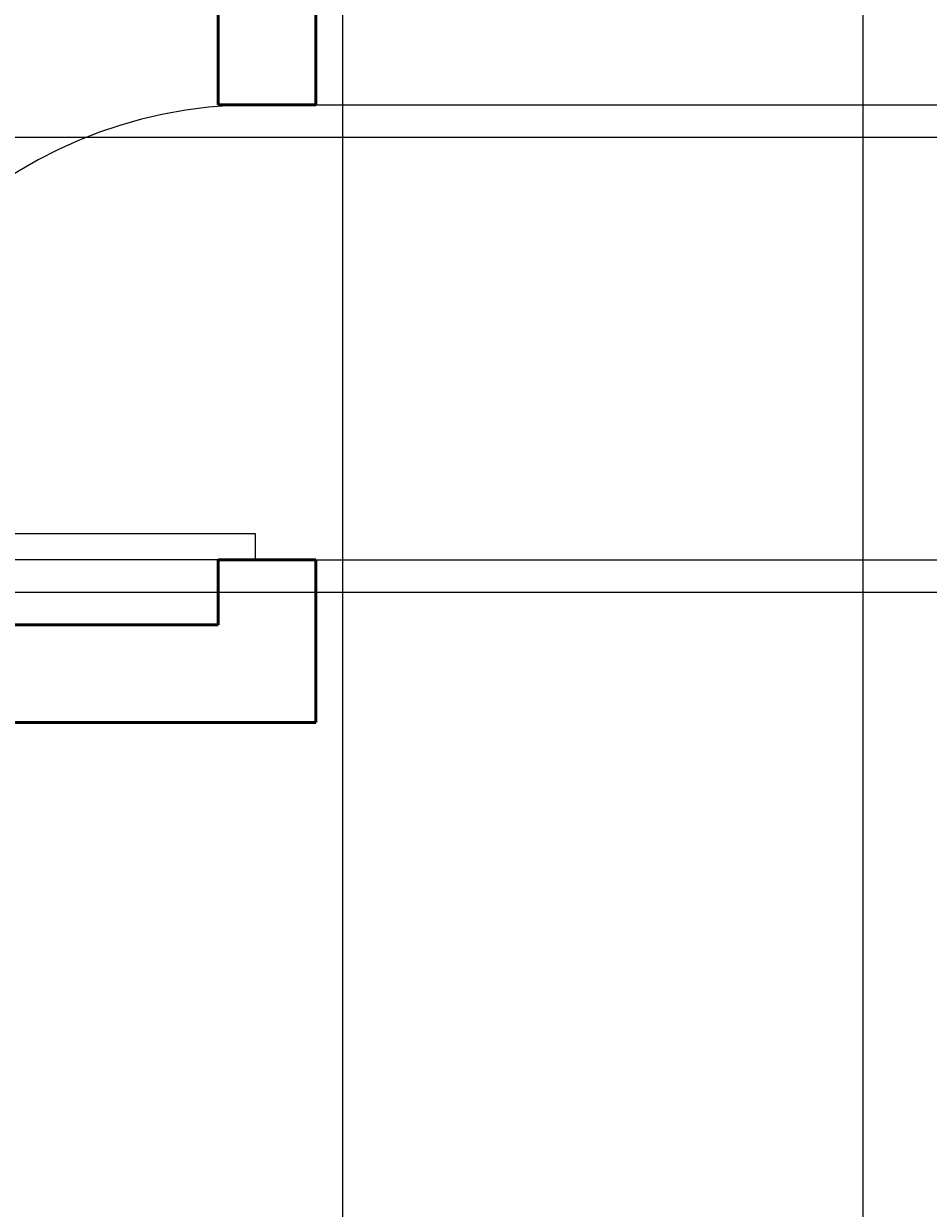
# Model space of a CAD drawing. Units: inches. Extents: x 5375 to 6084, y 16106 to 17259.
# Tile 24 of 32: x 5684 to 5768, y 16823 to 16932. Entities that reach past the tile are written whole.
import ezdxf

# ---------------------------------------------------------------- set-up
doc = ezdxf.new("R2010")
doc.units = ezdxf.units.IN
for name, color, linetype, lineweight in [('A-ANNO-DIMS', 2, 'Continuous', 18), ('DOOR', 4, 'Continuous', 25), ('WALL', 6, 'Continuous', 50)]:
    doc.layers.add(name, color=color, linetype=linetype, lineweight=lineweight)
doc.styles.get("Standard").update_dxf_attribs({"font": 'arial.ttf'})
doc.dimstyles.get("Standard").update_dxf_attribs({"dimtxt": 0.18, "dimasz": 0.18, "dimexe": 0.18, "dimexo": 0.0625, "dimgap": 0.09, "dimtad": 0, "dimtih": 1, "dimtoh": 1, "dimdec": 4, "dimzin": 0, "dimdsep": 46, "dimtxsty": 'Standard', "dimcen": 0.09, "dimadec": 0, "dimazin": 0, "dimtfac": 1, "dimtdec": 4, "dimtofl": 0, "dimtmove": 0, "dimatfit": 3, "dimfxl": 1, "dimtolj": 1, "dimtzin": 0, "dimarcsym": 0})

# ---------------------------------------------------------------- blocks, each defined once
blk = doc.blocks.new('*U2')
for p, q in [((0, 0), (0, -100)), ((750, 0), (750, -100))]:
    blk.add_line(p, q)
blk.add_lwpolyline([(0, 0), (0, 750), (43.75, 750), (43.75, 0)], close=True)
blk.add_arc((0, 0), 750, 0, 90)
blk = doc.blocks.new('*D39')
at = {"layer": 'A-ANNO-DIMS', "color": 0, "lineweight": -2, "transparency": 16777216}
for p, q in [((5713.62, 16402.64), (5713.62, 17259.16)), ((5761.62, 16402.64), (5761.62, 17259.16)), ((5713.8, 17258.98), (5737.4, 17258.98)), ((5761.44, 17258.98), (5737.84, 17258.98))]:
    blk.add_line(p, q, dxfattribs=at)
at = {"layer": 'A-ANNO-DIMS', "color": 0, "transparency": 16777216}
for points in [[(5713.8, 17259.01), (5713.8, 17258.95), (5713.62, 17258.98)], [(5761.44, 17259.01), (5761.44, 17258.95), (5761.62, 17258.98)]]:
    blk.add_solid(points, dxfattribs=at)
at = {"layer": 'Defpoints', "color": 0, "transparency": 16777216}
for p in [(5761.62, 17258.98), (5713.62, 16402.58), (5761.62, 16402.58)]:
    blk.add_point(p, dxfattribs=at)
at = {"layer": 'A-ANNO-DIMS', "color": 0, "transparency": 16777216, "insert": (5737.62, 17258.98), "char_height": 0.18, "attachment_point": 5}
blk.add_mtext('\\A1;48', dxfattribs=at)
blk = doc.blocks.new('*D41')
at = {"layer": 'A-ANNO-DIMS', "color": 0, "lineweight": -2, "transparency": 16777216}
for p, q in [((5702.18, 16924.58), (6084.2, 16924.58)), ((6084.02, 16924.4), (6084.02, 16903.76)), ((6084.02, 16882.76), (6084.02, 16903.4)), ((5702.18, 16882.58), (6084.2, 16882.58))]:
    blk.add_line(p, q, dxfattribs=at)
at = {"layer": 'A-ANNO-DIMS', "color": 0, "transparency": 16777216}
for points in [[(6083.99, 16924.4), (6084.05, 16924.4), (6084.02, 16924.58)], [(6083.99, 16882.76), (6084.05, 16882.76), (6084.02, 16882.58)]]:
    blk.add_solid(points, dxfattribs=at)
at = {"layer": 'Defpoints', "color": 0, "transparency": 16777216}
for p in [(5702.12, 16924.58), (6084.02, 16924.58), (5702.12, 16882.58)]:
    blk.add_point(p, dxfattribs=at)
at = {"layer": 'A-ANNO-DIMS', "color": 0, "transparency": 16777216, "insert": (6084.02, 16903.58), "char_height": 0.18, "attachment_point": 5}
blk.add_mtext('\\A1;42', dxfattribs=at)
blk = doc.blocks.new('*D42')
at = {"layer": 'A-ANNO-DIMS', "color": 0, "lineweight": -2, "transparency": 16777216}
for p, q in [((5826.06, 16921.58), (5375.56, 16921.58)), ((5375.74, 16921.4), (5375.74, 16900.76)), ((5375.74, 16879.76), (5375.74, 16900.4)), ((5826.06, 16879.58), (5375.56, 16879.58))]:
    blk.add_line(p, q, dxfattribs=at)
at = {"layer": 'A-ANNO-DIMS', "color": 0, "transparency": 16777216}
for points in [[(5375.71, 16921.4), (5375.77, 16921.4), (5375.74, 16921.58)], [(5375.71, 16879.76), (5375.77, 16879.76), (5375.74, 16879.58)]]:
    blk.add_solid(points, dxfattribs=at)
at = {"layer": 'Defpoints', "color": 0, "transparency": 16777216}
for p in [(5826.12, 16921.58), (5375.74, 16879.58), (5826.12, 16879.58)]:
    blk.add_point(p, dxfattribs=at)
at = {"layer": 'A-ANNO-DIMS', "color": 0, "transparency": 16777216, "insert": (5375.74, 16900.58), "char_height": 0.18, "attachment_point": 5}
blk.add_mtext('\\A1;42', dxfattribs=at)

msp = doc.modelspace()

# ---------------------------------------------------------------- linework, layer by layer
at = {"layer": 'WALL'}
for p, q in [((5702.1199, 17056.5793), (5702.1199, 16924.5793)), ((5711.1199, 17008.5793), (5711.1199, 16924.5793)), ((5702.1199, 16924.5793), (5711.1199, 16924.5793)), ((5702.1199, 16882.5793), (5711.1199, 16882.5793)), ((5702.1199, 16882.5793), (5702.1199, 16876.5793)), ((5711.1199, 16882.5793), (5711.1199, 16867.5793)), ((5529.6199, 16876.5793), (5702.1199, 16876.5793)), ((5553.6199, 16867.5793), (5711.1199, 16867.5793))]:
    msp.add_line(p, q, dxfattribs=at)

# ---------------------------------------------------------------- block references
at = {"layer": 'DOOR', "xscale": 0.0559999999999998, "yscale": 0.0559999999999998, "zscale": 0.0559999999999998, "rotation": 90.00000000000003}
msp.add_blockref('*U2', (5705.5199, 16882.5793), dxfattribs=at)

# ---------------------------------------------------------------- dimensions: what is measured, and where the dimension line sits
at = {"layer": 'A-ANNO-DIMS'}
dim = msp.add_linear_dim(base=(5761.6199, 17258.9793), p1=(5713.6199, 16402.5793), p2=(5761.6199, 16402.5793), dimstyle='Standard', override={"dimdec": 0, "dimlfac": 1, "dimrnd": 0, "dimzin": 0, "dimdsep": 46, "dimlunit": 2}, dxfattribs=at)
dim.commit()
dim.dimension.update_dxf_attribs({"geometry": '*D39', "text_midpoint": (5737.6199, 17258.9793)})
for base, p1, p2, picture, middle in [((6084.0199, 16924.5793), (5702.1199, 16882.5793), (5702.1199, 16924.5793), '*D41', (6084.0199, 16903.5793)), ((5375.7423, 16879.5793), (5826.1199, 16921.5793), (5826.1199, 16879.5793), '*D42', (5375.7423, 16900.5793))]:
    dim = msp.add_linear_dim(base=base, p1=p1, p2=p2, angle=90, dimstyle='Standard', override={"dimdec": 0, "dimlfac": 1, "dimrnd": 0, "dimzin": 0, "dimdsep": 46, "dimlunit": 2}, dxfattribs=at)
    dim.commit()
    dim.dimension.update_dxf_attribs({"geometry": picture, "text_midpoint": middle})

doc.saveas('drawing.dxf')
